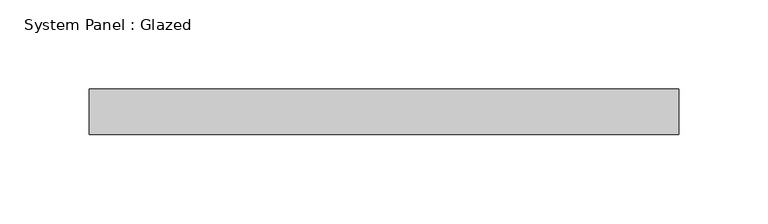
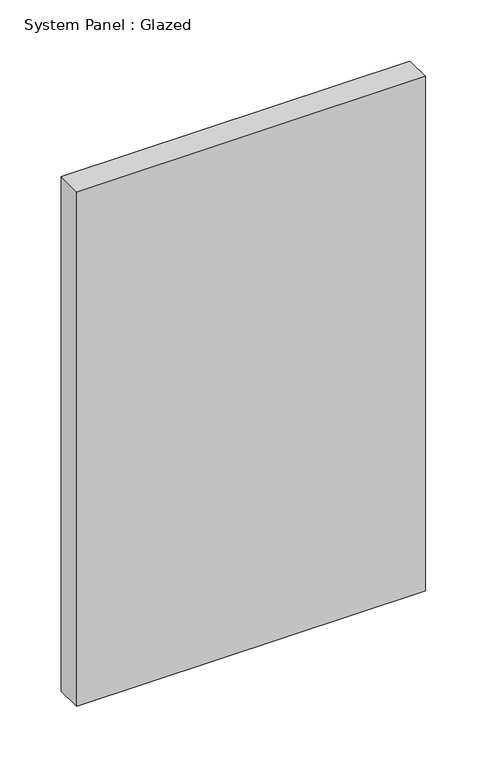
"""IFC4 building model written with IfcOpenShell, lengths in millimetres: plate geometry, System Panel : Glazed."""

from ifc_helpers import new_model, si_unit, origin, origin_with_axes, place, context, project, spatial, polyline, outline, extrude, source, transform, mapped, element, save


def system_panel_glazed_bfb04d77(model_context):
    return source(origin(), model_context, "Body", "SweptSolid", [
        extrude(outline(polyline([(165.1, 19.05), (-165.1, 19.05), (-165.1, 44.45), (165.1, 44.45), (165.1, 19.05)])), origin_with_axes(), (0.0, 0.0, 1.0), 514.35),
    ])


if __name__ == "__main__":
    model = new_model("IFC4")
    model_context = context("Model", 3, world=origin())
    ifc_project = project(units=[si_unit("LENGTHUNIT", "METRE", prefix="MILLI")], contexts=[model_context])
    site = spatial("IfcSite", under=ifc_project)
    building = spatial("IfcBuilding", under=site)
    placement = place(None, origin())
    system_panel_glazed_shape = system_panel_glazed_bfb04d77(model_context)
    element("IfcPlate", 1, ObjectType="System Panel : Glazed", at=placement, inside=building, context=model_context, shape_type="MappedRepresentation", body=[
        mapped(system_panel_glazed_shape, transform((0.0, 0.0, 0.0), x_axis=(1.0, 0.0, 0.0), y_axis=(0.0, 1.0, 0.0), z_axis=(0.0, 0.0, 1.0))),
    ])
    save(model, "model.ifc")

# Revit data of these elements
# Type "System Panel : Glazed"
#   Construction Type Id = "GSP4R"
#   Analytic Construction = "1/8 in Pilkington single glazing"
#   Visual Light Transmittance = 0.9
#   Solar Heat Gain Coefficient = 0.86
#   Heat Transfer Coefficient (U) = 1.18115 BTU/(h·ft²·°F)
#   Define Thermal Properties by = 1
# Element 1 (IfcPlate, "System Panel : Glazed")
#   Materials on its faces: "Glass"
# Materials
#   "Glass": class "Glass", colour RGB 0 128 192, transparency 0.75, Description = "Soda Lime Glass", Cost = 0
